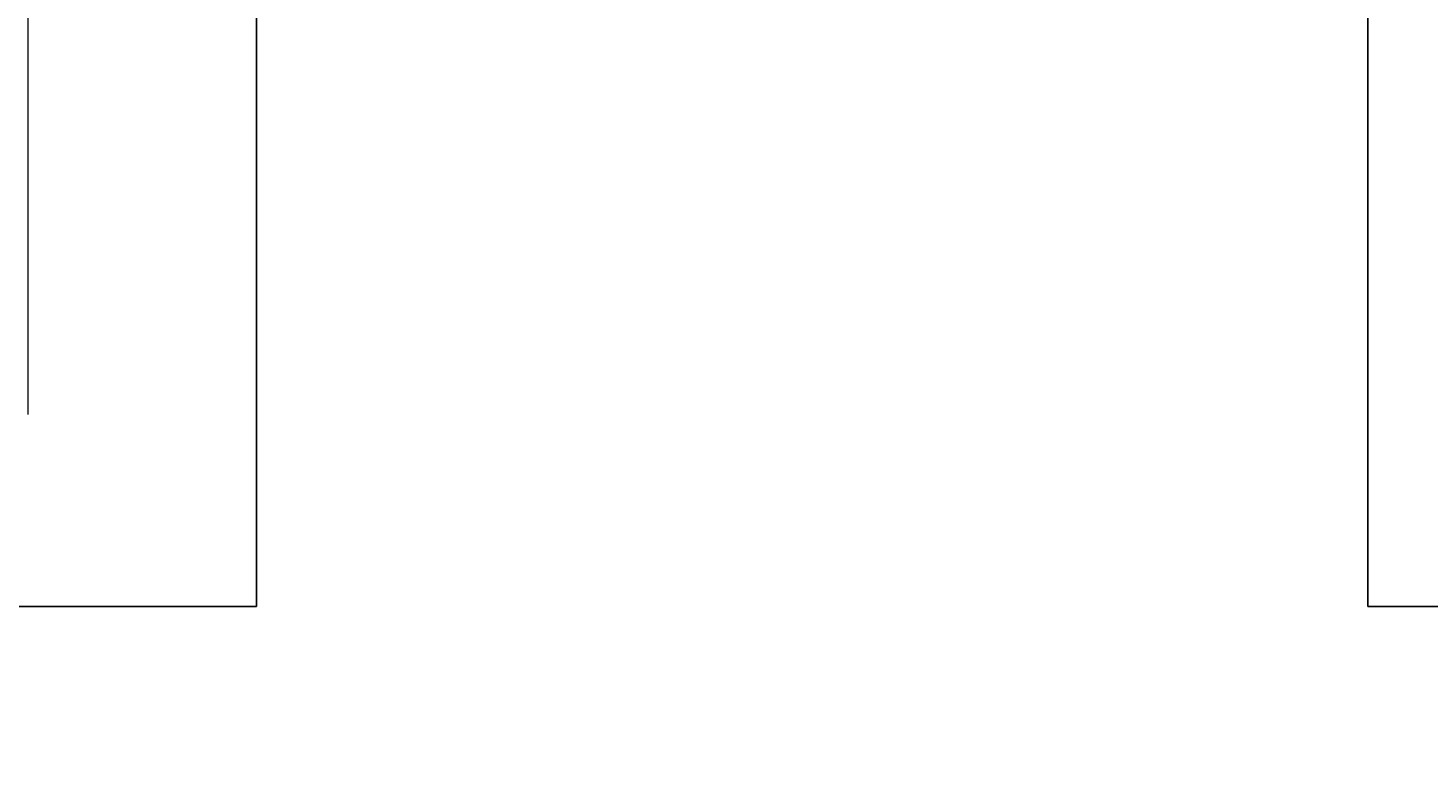
# Model space of a CAD drawing. Units: inches. Extents: x 1885 to 2748, y 783 to 2421.
# Tile 15 of 117: x 2102 to 2163, y 1050 to 1082. Entities that reach past the tile are written whole.
import ezdxf

# ---------------------------------------------------------------- set-up
doc = ezdxf.new("R2010")
doc.units = ezdxf.units.IN
for name, color, linetype, lineweight in [('A-ANNO-DIMS', 2, 'Continuous', 18), ('A-DOOR', 31, 'Continuous', 18), ('A-FLOR-BALC', 7, 'Continuous', 25)]:
    doc.layers.add(name, color=color, linetype=linetype, lineweight=lineweight)
doc.styles.get("Standard").update_dxf_attribs({"font": 'arial.ttf'})
doc.dimstyles.get("Standard").update_dxf_attribs({"dimtxt": 0.18, "dimasz": 0.18, "dimexe": 0.18, "dimexo": 0.0625, "dimgap": 0.09, "dimtad": 0, "dimtih": 1, "dimtoh": 1, "dimdec": 4, "dimzin": 0, "dimdsep": 46, "dimtxsty": 'Standard', "dimcen": 0.09, "dimadec": 0, "dimazin": 0, "dimtfac": 1, "dimtdec": 4, "dimtofl": 0, "dimtmove": 0, "dimatfit": 3, "dimfxl": 1, "dimtolj": 1, "dimtzin": 0, "dimarcsym": 0})

# ---------------------------------------------------------------- blocks, each defined once
blk = doc.blocks.new('*D43')
at = {"layer": 'A-ANNO-DIMS', "color": 0, "lineweight": -2, "transparency": 16777216}
for p, q in [((1971.274, 1057.443), (1971.274, 922.479)), ((2618.274, 1057.443), (2618.274, 922.479)), ((1971.454, 922.659), (2294.484, 922.659)), ((2618.094, 922.659), (2295.063, 922.659))]:
    blk.add_line(p, q, dxfattribs=at)
at = {"layer": 'A-ANNO-DIMS', "color": 0, "transparency": 16777216}
for points in [[(1971.454, 922.689), (1971.454, 922.629), (1971.274, 922.659)], [(2618.094, 922.689), (2618.094, 922.629), (2618.274, 922.659)]]:
    blk.add_solid(points, dxfattribs=at)
at = {"layer": 'Defpoints', "color": 0, "transparency": 16777216}
for p in [(1971.274, 1057.506), (2618.274, 1057.506), (2618.274, 922.659)]:
    blk.add_point(p, dxfattribs=at)
at = {"layer": 'A-ANNO-DIMS', "color": 0, "transparency": 16777216, "insert": (2294.774, 922.659), "char_height": 0.18, "attachment_point": 5}
blk.add_mtext('\\A1;647', dxfattribs=at)

msp = doc.modelspace()

# ---------------------------------------------------------------- linework, layer by layer
at = {"layer": 'A-DOOR'}
msp.add_line((2102.465, 1089.756), (2102.465, 1065.756), dxfattribs=at)
at = {"layer": 'A-FLOR-BALC'}
for p, q in [((2112.274, 1057.506), (2112.274, 1087.506)), ((2159.936, 1087.506), (2159.936, 1057.506)), ((1971.274, 1057.506), (2112.274, 1057.506)), ((2159.936, 1057.506), (2301.274, 1057.506))]:
    msp.add_line(p, q, dxfattribs=at)

# ---------------------------------------------------------------- dimensions: what is measured, and where the dimension line sits
at = {"layer": 'A-ANNO-DIMS'}
dim = msp.add_linear_dim(base=(2618.274, 922.659), p1=(1971.274, 1057.506), p2=(2618.274, 1057.506), dimstyle='Standard', override={"dimdec": 0, "dimlfac": 1, "dimrnd": 0, "dimzin": 0, "dimdsep": 46, "dimlunit": 2}, dxfattribs=at)
dim.commit()
dim.dimension.update_dxf_attribs({"geometry": '*D43', "text_midpoint": (2294.774, 922.659)})

doc.saveas('drawing.dxf')
